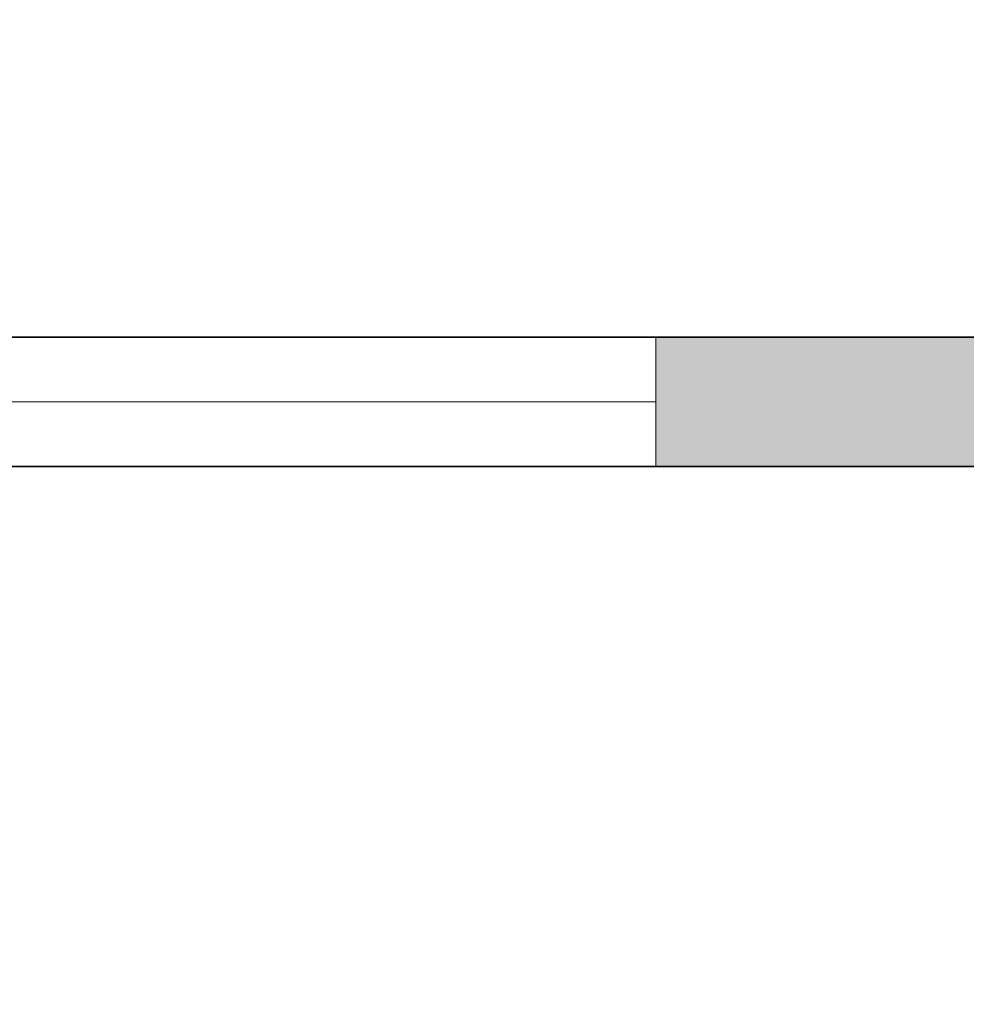
# Model space of a CAD drawing. Units: inches. Extents: x 1319 to 2030, y 219 to 1069.
# Tile 19 of 28: x 1499 to 1565, y 515 to 583. Entities that reach past the tile are written whole.
import ezdxf

# ---------------------------------------------------------------- set-up
doc = ezdxf.new("R2010")
doc.units = ezdxf.units.IN
doc.header["$MEASUREMENT"] = 0
for name, color, linetype, lineweight in [('A-GLAZ', 4, 'Continuous', 18), ('A-WALL-PATT', 252, 'Continuous', 13), ('walls', 250, 'Continuous', 35)]:
    doc.layers.add(name, color=color, linetype=linetype, lineweight=lineweight)

msp = doc.modelspace()

# ---------------------------------------------------------------- hatches: boundary and pattern name
at = {"layer": 'A-WALL-PATT'}
h = msp.add_hatch(color=256, dxfattribs=at)
h.dxf.hatch_style = 1
h.paths.add_polyline_path([(1856.292, 860.616), (1812.343, 860.616), (1812.343, 851.616), (1812.343, 700.993), (1816.843, 700.993), (1816.843, 851.616), (1856.292, 851.616)])
h.paths.add_polyline_path([(1960.843, 663.616), (1812.343, 663.616), (1782.783, 663.616), (1782.783, 659.116), (1812.343, 659.116), (1960.843, 659.116)])
h.paths.add_polyline_path([(1857.424, 659.116), (1852.924, 659.116), (1852.924, 616.807), (1857.424, 616.807)])
h.paths.add_polyline_path([(1735.843, 661.727), (1731.843, 661.727), (1636.133, 661.727), (1636.133, 657.227), (1731.343, 657.227), (1731.343, 481.227), (1618.616, 481.227), (1618.616, 472.227), (1639.343, 472.227), (1639.343, 384.227), (1627.044, 384.227), (1627.044, 375.227), (1648.343, 375.227), (1648.343, 384.227), (1648.343, 472.227), (1750.706, 472.227), (1750.706, 481.227), (1735.843, 481.227), (1735.843, 657.727)])
h.paths.add_polyline_path([(1587.343, 481.227), (1578.343, 481.227), (1578.343, 375.227), (1597.622, 375.227), (1597.622, 384.227), (1587.343, 384.227)])
h.paths.add_polyline_path([(1769.593, 384.227), (1693.482, 384.227), (1693.482, 375.227), (1769.593, 375.227)])
h.paths.add_polyline_path([(1775.828, 481.227), (1765.831, 481.227), (1765.831, 472.227), (1775.828, 472.227)])
h.paths.add_polyline_path([(1824.625, 481.227), (1820.343, 481.227), (1820.343, 476.727), (1824.625, 476.727), (1824.625, 477.545)], flags=0)
h.paths.add_polyline_path([(1896.843, 481.227), (1852.26, 481.227), (1852.26, 476.727), (1892.343, 476.727), (1892.343, 384.227), (1881.742, 384.227), (1881.742, 375.227), (1913.435, 375.227), (1913.435, 384.227), (1896.843, 384.227)])
h.paths.add_polyline_path([(1960.843, 481.227), (1931.341, 481.227), (1931.341, 476.727), (1960.843, 476.727)])
h.paths.add_polyline_path([(1736.343, 918.227), (1731.843, 918.227), (1731.843, 890.227), (1582.843, 890.227), (1582.843, 781.727), (1582.843, 769.171), (1587.343, 769.171), (1587.343, 781.727), (1587.343, 885.727), (1731.843, 885.727), (1731.843, 851.616), (1736.343, 851.616), (1736.343, 890.227)])
h.paths.add_polyline_path([(1781.022, 860.616), (1773.021, 860.616, -0.032228), (1773.289, 856.464), (1773.289, 851.616), (1781.022, 851.616)])
h.paths.add_polyline_path([(1587.343, 946.227), (1582.843, 946.227), (1582.843, 926.136), (1587.343, 926.136)])
h.paths.add_polyline_path([(1647.843, 946.227), (1643.343, 946.227), (1643.343, 926.136), (1647.843, 926.136)])
h.paths.add_polyline_path([(1543.343, 786.227), (1429.843, 786.227), (1429.843, 757.555), (1434.343, 757.555), (1438.843, 757.555), (1438.843, 781.727), (1543.343, 781.727)])
h.paths.add_polyline_path([(1543.343, 781.727), (1538.843, 781.727), (1538.843, 709.727), (1534.597, 709.727), (1534.597, 705.227), (1543.343, 705.227), (1543.343, 709.727)])
h.paths.add_polyline_path([(1499.955, 709.727), (1438.843, 709.727), (1438.843, 734.463), (1429.843, 734.463), (1429.843, 552.227), (1470.241, 552.227), (1470.241, 561.227), (1438.843, 561.227), (1438.843, 705.227), (1499.955, 705.227)])
h.paths.add_polyline_path([(1587.343, 709.727), (1582.843, 709.727), (1582.843, 561.227), (1543.433, 561.227), (1543.433, 552.227), (1587.343, 552.227)])
h.paths.add_polyline_path([(1546.835, 709.727), (1543.343, 709.727), (1543.343, 705.227), (1546.835, 705.227)])
h.paths.add_polyline_path([(1582.843, 709.727), (1579.15, 709.727), (1579.15, 705.227), (1582.843, 705.227)], flags=17)
h.paths.add_polyline_path([(1548.368, 786.227), (1543.343, 786.227), (1543.343, 781.727), (1548.368, 781.727)])
h.paths.add_polyline_path([(1582.843, 786.227), (1580.683, 786.227), (1580.683, 781.727), (1582.843, 781.727)])
h.paths.add_polyline_path([(1587.343, 892.402), (1582.843, 892.402), (1582.843, 890.227), (1587.343, 890.227)], flags=17)
h.paths.add_polyline_path([(1647.843, 892.402), (1643.343, 892.402), (1643.343, 890.227), (1647.843, 890.227)], flags=17)
h.paths.add_polyline_path([(1740.974, 856.464), (1740.974, 860.616), (1736.343, 860.616), (1736.343, 851.616), (1740.974, 851.616)])
h.paths.add_polyline_path([(1853.989, 384.227), (1820.343, 384.227), (1820.343, 402.924), (1815.843, 402.924), (1815.843, 375.227), (1853.989, 375.227)])
h.paths.add_polyline_path([(1892.343, 436.227), (1820.343, 436.227), (1820.343, 481.227), (1815.843, 481.227), (1815.843, 431.727), (1892.343, 431.727)])
h.paths.add_polyline_path([(1849.175, 481.227), (1824.625, 481.227), (1824.625, 477.545), (1825.699, 477.545), (1825.699, 453.018, 0.401453), (1849.175, 477.545)], flags=0)
h.paths.add_polyline_path([(1960.843, 384.227), (1941.188, 384.227), (1941.188, 375.227), (1960.843, 375.227)])
h.paths.add_polyline_path([(1902.267, 481.227), (1896.843, 481.227), (1896.843, 476.727), (1902.267, 476.727), (1902.267, 477.44)], flags=0)

# ---------------------------------------------------------------- linework, layer by layer
at = {"layer": 'A-GLAZ'}
for p, q in [((1543.433, 561.227), (1470.241, 561.227)), ((1543.433, 552.227), (1543.433, 561.227)), ((1470.241, 556.727), (1543.433, 556.727)), ((1470.241, 552.227), (1543.433, 552.227))]:
    msp.add_line(p, q, dxfattribs=at)
at = {"layer": 'walls'}
for p, q in [((1438.843, 561.227), (1582.843, 561.227)), ((1429.843, 552.227), (1587.343, 552.227))]:
    msp.add_line(p, q, dxfattribs=at)

doc.saveas('drawing.dxf')
